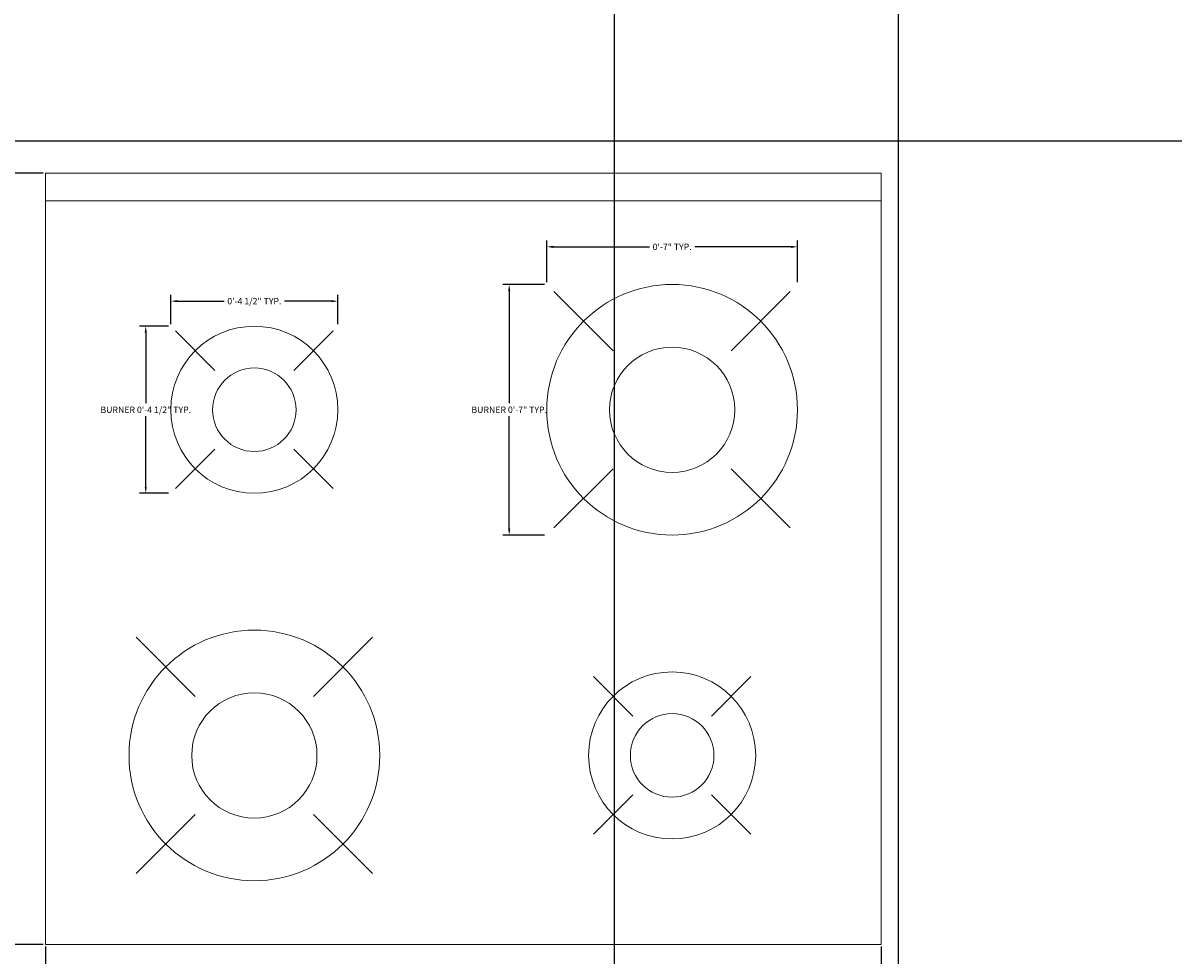
# Model space of a CAD drawing. Units: inches. Extents: x -5 to 330, y -522 to 40.
# Tile 6 of 23: x 62 to 95, y -417 to -391. Entities that reach past the tile are written whole.
import ezdxf

# ---------------------------------------------------------------- set-up
doc = ezdxf.new("R2010")
doc.units = ezdxf.units.IN
doc.header["$MEASUREMENT"] = 0
for name, color, linetype, lineweight in [('A-ANNO-DIMS', 2, 'Continuous', 18), ('A-EQPM', 8, 'Continuous', 18), ('A-FLOR-CASE', 8, 'Continuous', 25)]:
    doc.layers.add(name, color=color, linetype=linetype, lineweight=lineweight)
doc.styles.get("Standard").update_dxf_attribs({"font": 'arial.ttf'})
doc.dimstyles.get("Standard").update_dxf_attribs({"dimtxt": 0.18, "dimasz": 0.18, "dimexe": 0.18, "dimexo": 0.0625, "dimgap": 0.09, "dimtad": 0, "dimtih": 1, "dimtoh": 1, "dimdec": 0, "dimzin": 0, "dimdsep": 46, "dimlunit": 3, "dimtxsty": 'Standard', "dimcen": 0.09, "dimadec": 0, "dimazin": 0, "dimtfac": 1, "dimtdec": 0, "dimtofl": 0, "dimtmove": 0, "dimatfit": 3, "dimfxl": 1, "dimtolj": 1, "dimtzin": 0, "dimarcsym": 0})

# ---------------------------------------------------------------- blocks, each defined once
blk = doc.blocks.new('COOKTOP-BURNER-LARGE')
for p, q in [((1.865, 5.19), (0.202, 6.852)), ((5.19, 5.19), (6.853, 6.852)), ((1.865, 1.864), (0.202, 0.202)), ((5.19, 1.864), (6.853, 0.202))]:
    blk.add_line(p, q)
blk.add_circle((3.527, 3.527), 3.527)
for start, end in [(0, 180), (180, 0)]:
    blk.add_arc((3.527, 3.527), 1.763, start, end)
blk = doc.blocks.new('COOKTOP-BURNER-SMALL')
for p, q in [((1.243, 3.46), (0.134, 4.568)), ((3.46, 3.46), (4.568, 4.568)), ((1.243, 1.243), (0.134, 0.134)), ((3.46, 1.243), (4.568, 0.134))]:
    blk.add_line(p, q)
blk.add_circle((2.351, 2.351), 2.351)
for start, end in [(0, 180), (180, 0)]:
    blk.add_arc((2.351, 2.351), 1.176, start, end)
blk = doc.blocks.new('*D29')
at = {"layer": 'A-ANNO-DIMS', "color": 0, "lineweight": -2, "transparency": 16777216}
for p, q in [((77.055, -397.969), (75.88, -397.969)), ((76.06, -398.149), (76.06, -401.314)), ((76.06, -404.843), (76.06, -401.678)), ((77.055, -405.023), (75.88, -405.023))]:
    blk.add_line(p, q, dxfattribs=at)
at = {"layer": 'A-ANNO-DIMS', "color": 0, "transparency": 16777216}
for points in [[(76.03, -398.149), (76.09, -398.149), (76.06, -397.969)], [(76.03, -404.843), (76.09, -404.843), (76.06, -405.023)]]:
    blk.add_solid(points, dxfattribs=at)
at = {"layer": 'Defpoints', "color": 0, "transparency": 16777216}
for p in [(77.118, -397.969), (76.06, -405.023), (77.118, -405.023)]:
    blk.add_point(p, dxfattribs=at)
at = {"layer": 'A-ANNO-DIMS', "color": 0, "transparency": 16777216, "insert": (76.06, -401.496), "char_height": 0.18, "attachment_point": 5}
blk.add_mtext('\\A1;BURNER 0\'-7" TYP.', dxfattribs=at)
blk = doc.blocks.new('*D30')
at = {"layer": 'A-ANNO-DIMS', "color": 0, "lineweight": -2, "transparency": 16777216}
for p, q in [((77.118, -397.906), (77.118, -396.731)), ((84.172, -397.906), (84.172, -396.731)), ((77.298, -396.911), (80.006, -396.911)), ((83.992, -396.911), (81.283, -396.911))]:
    blk.add_line(p, q, dxfattribs=at)
at = {"layer": 'A-ANNO-DIMS', "color": 0, "transparency": 16777216}
for points in [[(77.298, -396.881), (77.298, -396.941), (77.118, -396.911)], [(83.992, -396.881), (83.992, -396.941), (84.172, -396.911)]]:
    blk.add_solid(points, dxfattribs=at)
at = {"layer": 'Defpoints', "color": 0, "transparency": 16777216}
for p in [(77.118, -396.911), (77.118, -397.969), (84.172, -397.969)]:
    blk.add_point(p, dxfattribs=at)
at = {"layer": 'A-ANNO-DIMS', "color": 0, "transparency": 16777216, "insert": (80.645, -396.911), "char_height": 0.18, "attachment_point": 5}
blk.add_mtext('\\A1;0\'-7" TYP.', dxfattribs=at)
blk = doc.blocks.new('*D31')
at = {"layer": 'A-ANNO-DIMS', "color": 0, "lineweight": -2, "transparency": 16777216}
for p, q in [((66.475, -399.144), (65.652, -399.144)), ((65.832, -399.324), (65.832, -401.313)), ((65.832, -403.667), (65.832, -401.679)), ((66.475, -403.847), (65.652, -403.847))]:
    blk.add_line(p, q, dxfattribs=at)
at = {"layer": 'A-ANNO-DIMS', "color": 0, "transparency": 16777216}
for points in [[(65.802, -399.324), (65.862, -399.324), (65.832, -399.144)], [(65.802, -403.667), (65.862, -403.667), (65.832, -403.847)]]:
    blk.add_solid(points, dxfattribs=at)
at = {"layer": 'Defpoints', "color": 0, "transparency": 16777216}
for p in [(65.832, -399.144), (66.537, -399.144), (66.537, -403.847)]:
    blk.add_point(p, dxfattribs=at)
at = {"layer": 'A-ANNO-DIMS', "color": 0, "transparency": 16777216, "insert": (65.832, -401.496), "char_height": 0.18, "attachment_point": 5}
blk.add_mtext('\\A1;BURNER 0\'-4 1/2" TYP.', dxfattribs=at)
blk = doc.blocks.new('*D32')
at = {"layer": 'A-ANNO-DIMS', "color": 0, "lineweight": -2, "transparency": 16777216}
for p, q in [((66.537, -399.082), (66.537, -398.259)), ((71.24, -399.082), (71.24, -398.259)), ((66.717, -398.439), (68.04, -398.439)), ((71.06, -398.439), (69.737, -398.439))]:
    blk.add_line(p, q, dxfattribs=at)
at = {"layer": 'A-ANNO-DIMS', "color": 0, "transparency": 16777216}
for points in [[(66.717, -398.409), (66.717, -398.469), (66.537, -398.439)], [(71.06, -398.409), (71.06, -398.469), (71.24, -398.439)]]:
    blk.add_solid(points, dxfattribs=at)
at = {"layer": 'Defpoints', "color": 0, "transparency": 16777216}
for p in [(71.24, -398.439), (66.537, -399.144), (71.24, -399.144)]:
    blk.add_point(p, dxfattribs=at)
at = {"layer": 'A-ANNO-DIMS', "color": 0, "transparency": 16777216, "insert": (68.888, -398.439), "char_height": 0.18, "attachment_point": 5}
blk.add_mtext('\\A1;0\'-4 1/2" TYP.', dxfattribs=at)
blk = doc.blocks.new('*D40')
at = {"layer": 'A-ANNO-DIMS', "color": 0, "lineweight": -2, "transparency": 16777216}
for p, q in [((32.51, -246.706), (32.51, -522.309)), ((79.01, -246.706), (79.01, -522.309)), ((32.69, -522.129), (55.151, -522.129)), ((78.83, -522.129), (56.369, -522.129))]:
    blk.add_line(p, q, dxfattribs=at)
at = {"layer": 'A-ANNO-DIMS', "color": 0, "transparency": 16777216}
for points in [[(32.69, -522.099), (32.69, -522.159), (32.51, -522.129)], [(78.83, -522.099), (78.83, -522.159), (79.01, -522.129)]]:
    blk.add_solid(points, dxfattribs=at)
at = {"layer": 'Defpoints', "color": 0, "transparency": 16777216}
for p in [(32.51, -246.644), (79.01, -246.644), (79.01, -522.129)]:
    blk.add_point(p, dxfattribs=at)
at = {"layer": 'A-ANNO-DIMS', "color": 0, "transparency": 16777216, "insert": (55.76, -522.129), "char_height": 0.18, "attachment_point": 5}
blk.add_mtext('\\A1;3\'-10 1/2"', dxfattribs=at)
blk = doc.blocks.new('*D41')
at = {"layer": 'A-ANNO-DIMS', "color": 0, "lineweight": -2, "transparency": 16777216}
for p, q in [((87.01, -246.706), (87.01, -522.309)), ((129.01, -246.706), (129.01, -522.309)), ((87.19, -522.129), (107.681, -522.129)), ((128.83, -522.129), (108.339, -522.129))]:
    blk.add_line(p, q, dxfattribs=at)
at = {"layer": 'A-ANNO-DIMS', "color": 0, "transparency": 16777216}
for points in [[(87.19, -522.099), (87.19, -522.159), (87.01, -522.129)], [(128.83, -522.099), (128.83, -522.159), (129.01, -522.129)]]:
    blk.add_solid(points, dxfattribs=at)
at = {"layer": 'Defpoints', "color": 0, "transparency": 16777216}
for p in [(87.01, -246.644), (129.01, -246.644), (129.01, -522.129)]:
    blk.add_point(p, dxfattribs=at)
at = {"layer": 'A-ANNO-DIMS', "color": 0, "transparency": 16777216, "insert": (108.01, -522.129), "char_height": 0.18, "attachment_point": 5}
blk.add_mtext('\\A1;3\'-6"', dxfattribs=at)
blk = doc.blocks.new('*D48')
at = {"layer": 'A-ANNO-DIMS', "color": 0, "lineweight": -2, "transparency": 16777216}
for p, q in [((63.01, -416.607), (63.01, -522.309)), ((86.523, -416.607), (86.523, -522.309)), ((63.19, -522.129), (74.166, -522.129)), ((86.343, -522.129), (75.367, -522.129))]:
    blk.add_line(p, q, dxfattribs=at)
at = {"layer": 'A-ANNO-DIMS', "color": 0, "transparency": 16777216}
for points in [[(63.19, -522.099), (63.19, -522.159), (63.01, -522.129)], [(86.343, -522.099), (86.343, -522.159), (86.523, -522.129)]]:
    blk.add_solid(points, dxfattribs=at)
at = {"layer": 'Defpoints', "color": 0, "transparency": 16777216}
for p in [(63.01, -416.544), (86.523, -416.544), (86.523, -522.129)]:
    blk.add_point(p, dxfattribs=at)
at = {"layer": 'A-ANNO-DIMS', "color": 0, "transparency": 16777216, "insert": (74.767, -522.129), "char_height": 0.18, "attachment_point": 5}
blk.add_mtext('\\A1;1\'-11 1/2"', dxfattribs=at)
blk = doc.blocks.new('*D49')
at = {"layer": 'A-ANNO-DIMS', "color": 0, "lineweight": -2, "transparency": 16777216}
for p, q in [((62.948, -394.834), (-3.655, -394.834)), ((-3.475, -395.014), (-3.475, -405.506)), ((-3.475, -416.364), (-3.475, -405.872)), ((62.948, -416.544), (-3.655, -416.544))]:
    blk.add_line(p, q, dxfattribs=at)
at = {"layer": 'A-ANNO-DIMS', "color": 0, "transparency": 16777216}
for points in [[(-3.505, -395.014), (-3.445, -395.014), (-3.475, -394.834)], [(-3.505, -416.364), (-3.445, -416.364), (-3.475, -416.544)]]:
    blk.add_solid(points, dxfattribs=at)
at = {"layer": 'Defpoints', "color": 0, "transparency": 16777216}
for p in [(63.01, -394.834), (-3.475, -416.544), (63.01, -416.544)]:
    blk.add_point(p, dxfattribs=at)
at = {"layer": 'A-ANNO-DIMS', "color": 0, "transparency": 16777216, "insert": (-3.475, -405.689), "char_height": 0.18, "attachment_point": 5}
blk.add_mtext('\\A1;1\'-9 1/2"', dxfattribs=at)

msp = doc.modelspace()

# ---------------------------------------------------------------- linework, layer by layer
at = {"layer": 'A-EQPM'}
for p, q in [((63.01, -394.834), (86.523, -394.834)), ((63.01, -394.834), (63.01, -416.544)), ((86.523, -394.834), (86.523, -416.544)), ((63.01, -395.618), (86.523, -395.618)), ((63.01, -416.544), (86.523, -416.544))]:
    msp.add_line(p, q, dxfattribs=at)
at = {"layer": 'A-FLOR-CASE'}
msp.add_line((48.129, -393.928), (128.51, -393.928), dxfattribs=at)

# ---------------------------------------------------------------- block references
at = {"layer": 'A-EQPM', "rotation": 180}
for name, p in [('COOKTOP-BURNER-LARGE', (84.172, -397.969)), ('COOKTOP-BURNER-SMALL', (82.996, -408.875))]:
    msp.add_blockref(name, p, dxfattribs=at)
at = {"layer": 'A-EQPM'}
for name, p in [('COOKTOP-BURNER-SMALL', (66.537, -403.847)), ('COOKTOP-BURNER-LARGE', (65.361, -414.753))]:
    msp.add_blockref(name, p, dxfattribs=at)

# ---------------------------------------------------------------- dimensions: what is measured, and where the dimension line sits
at = {"layer": 'A-ANNO-DIMS'}
for base, p1, p2, picture, middle in [((79.01, -522.129), (32.51, -246.644), (79.01, -246.644), '*D40', (55.76, -522.129)), ((129.01, -522.129), (87.01, -246.644), (129.01, -246.644), '*D41', (108.01, -522.129)), ((86.523, -522.129), (63.01, -416.544), (86.523, -416.544), '*D48', (74.767, -522.129))]:
    dim = msp.add_linear_dim(base=base, p1=p1, p2=p2, dimstyle='Standard', override={"dimdec": 1, "dimlfac": 1, "dimrnd": 0, "dimzin": 1, "dimdsep": 46, "dimlunit": 4, "dimfrac": 2}, dxfattribs=at)
    dim.commit()
    dim.dimension.update_dxf_attribs({"geometry": picture, "text_midpoint": middle})
dim = msp.add_linear_dim(base=(-3.475, -416.544), p1=(63.01, -394.834), p2=(63.01, -416.544), angle=90, dimstyle='Standard', override={"dimdec": 1, "dimlfac": 1, "dimrnd": 0, "dimzin": 1, "dimdsep": 46, "dimlunit": 4, "dimfrac": 2}, dxfattribs=at)
dim.commit()
dim.dimension.update_dxf_attribs({"geometry": '*D49', "text_midpoint": (-3.475, -405.689)})
for base, p1, p2, angle, text, picture, middle in [((77.118, -396.911), (84.172, -397.969), (77.118, -397.969), 180, '<> TYP.', '*D30', (80.645, -396.911)), ((76.06, -405.023), (77.118, -397.969), (77.118, -405.023), 270, 'BURNER <> TYP.', '*D29', (76.06, -401.496)), ((65.832, -399.144), (66.537, -403.847), (66.537, -399.144), 90, 'BURNER <> TYP.', '*D31', (65.832, -401.496))]:
    dim = msp.add_linear_dim(base=base, p1=p1, p2=p2, angle=angle, text=text, dimstyle='Standard', override={"dimdec": 1, "dimlfac": 1, "dimrnd": 0, "dimzin": 1, "dimdsep": 46, "dimlunit": 4, "dimfrac": 2}, dxfattribs=at)
    dim.commit()
    dim.dimension.update_dxf_attribs({"geometry": picture, "text_midpoint": middle})
dim = msp.add_linear_dim(base=(71.24, -398.439), p1=(66.537, -399.144), p2=(71.24, -399.144), text='<> TYP.', dimstyle='Standard', override={"dimdec": 1, "dimlfac": 1, "dimrnd": 0, "dimzin": 1, "dimdsep": 46, "dimlunit": 4, "dimfrac": 2}, dxfattribs=at)
dim.commit()
dim.dimension.update_dxf_attribs({"geometry": '*D32', "text_midpoint": (68.888, -398.439)})

doc.saveas('drawing.dxf')
